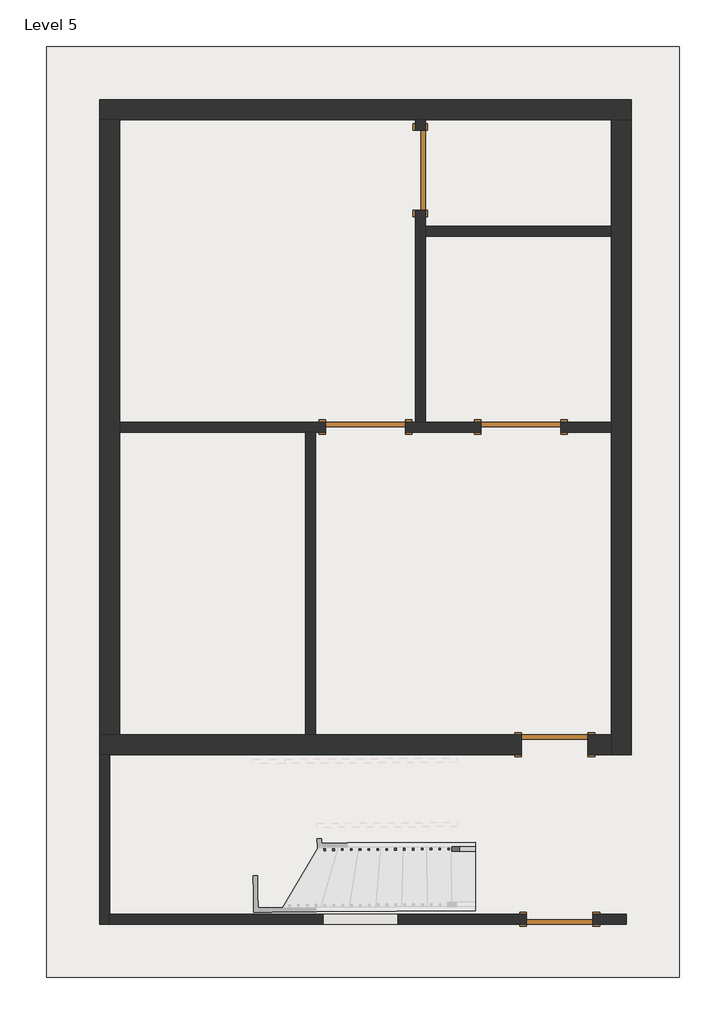
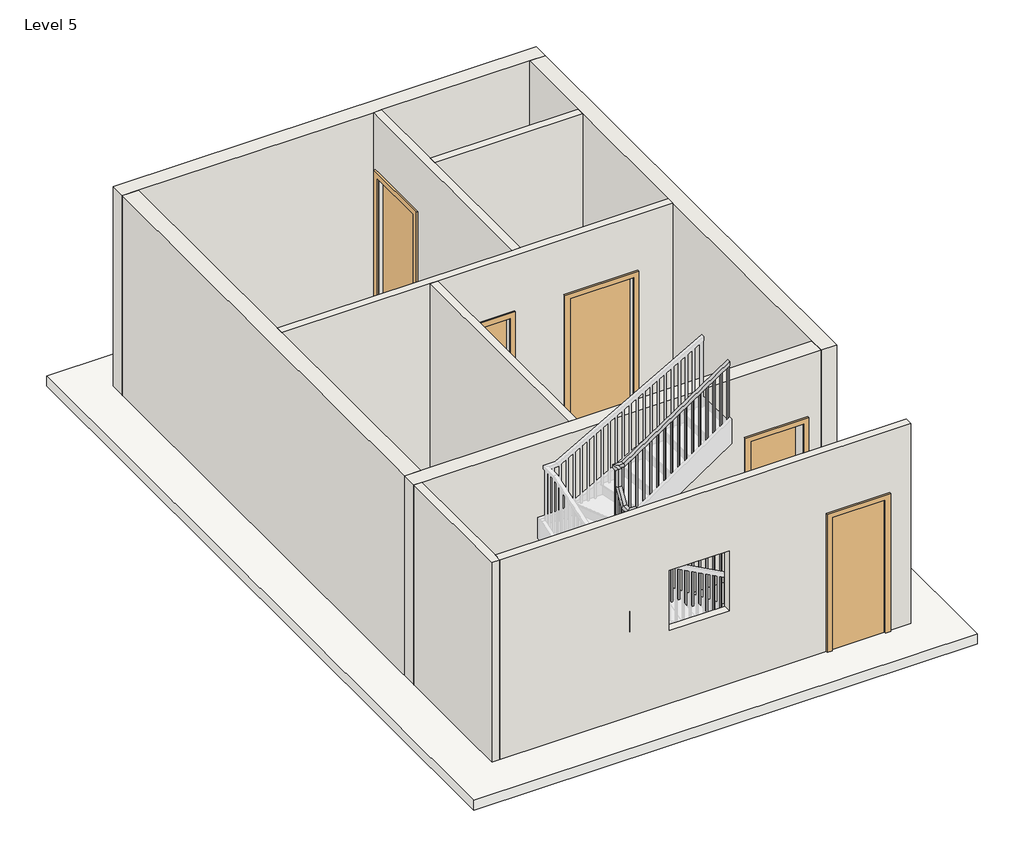
# One storey, part 1 of 2: 10 walls, 5 doors, 1 railing, 1 roof.
"""IFC4 building model written with IfcOpenShell, lengths in millimetres."""

from ifc_helpers import new_model, si_unit, frame, origin, place, context, project, spatial, polyline, outline, extrude, faceted_brep, transform, mapped, element, save
from components import door_a1484949, door_d8f5dbb5, door_e5f9f3c4, door_305aa2a5

model = new_model("IFC4")

# Units and contexts
model_context = context("Model", 3, world=origin())
ifc_project = project(units=[si_unit("LENGTHUNIT", "METRE", prefix="MILLI")], contexts=[model_context])

# Site, building, storey
site = spatial("IfcSite", under=ifc_project)
building = spatial("IfcBuilding", under=site)
storey = spatial("IfcBuildingStorey", under=building, Name="Level 5", Elevation=9601.2)

# Doors
placement = place(None, origin())
door_shape = door_a1484949(model_context)
element("IfcDoor", 1, ObjectType="Single-Flush : 30\" x 80\"", at=placement, inside=storey, context=model_context, shape_type="MappedRepresentation", body=[
    mapped(door_shape, transform((792.5410386, -2372.0109248, 9601.2), x_axis=(1.0, 0.0, 0.0), y_axis=(0.0, 1.0, 0.0), z_axis=(0.0, 0.0, 1.0))),
])
door_2_shape = door_d8f5dbb5(model_context)
element("IfcDoor", 2, ObjectType="Single-Flush : 30\" x 80\"", at=placement, inside=storey, context=model_context, shape_type="MappedRepresentation", body=[
    mapped(door_2_shape, transform((849.6910386, -4372.2609248, 9601.2), x_axis=(-1.0, 0.0, 0.0), y_axis=(0.0, -1.0, 0.0), z_axis=(0.0, 0.0, 1.0))),
])
door_3_shape = door_e5f9f3c4(model_context)
element("IfcDoor", 3, ObjectType="Single-Flush : 36\" x 84\"", at=placement, inside=storey, context=model_context, shape_type="MappedRepresentation", body=[
    mapped(door_3_shape, transform((-750.5089614, 4209.7640752, 9601.2), x_axis=(0.0, -1.0, 0.0), y_axis=(1.0, 0.0, 0.0), z_axis=(0.0, 0.0, 1.0))),
])
door_4_shape = door_305aa2a5(model_context)
element("IfcDoor", 4, ObjectType="Single-Flush : 36\" x 84\"", at=placement, inside=storey, context=model_context, shape_type="MappedRepresentation", body=[
    mapped(door_4_shape, transform((402.0160386, 1266.5390752, 9601.2), x_axis=(-1.0, 0.0, 0.0), y_axis=(0.0, -1.0, 0.0), z_axis=(0.0, 0.0, 1.0))),
])
element("IfcDoor", 5, ObjectType="Single-Flush : 36\" x 84\"", at=placement, inside=storey, context=model_context, shape_type="MappedRepresentation", body=[
    mapped(door_4_shape, transform((-1379.1589614, 1266.5390752, 9601.2), x_axis=(-1.0, 0.0, 0.0), y_axis=(0.0, -1.0, 0.0), z_axis=(0.0, 0.0, 1.0))),
])

# Railing
element("IfcRailing", 6, ObjectType="Handrail - Rectangular", at=placement, inside=storey, context=model_context, shape_type="SolidModel", body=[
    faceted_brep([(-120.3816305, -3590.4209536, 10684.9333333), (-120.3816305, -3590.4209536, 10623.7630107), (-120.6930289, -3539.621908, 10623.7630107), (-120.6930289, -3539.621908, 10684.9333333), (-1854.5612186, -3601.0514854, 11848.2182998), (-1905.3602642, -3601.3628839, 11821.1238978), (-1905.6716627, -3550.5638383, 11821.1238978), (-1854.8726171, -3550.2524399, 11848.2182998), (-1854.5612186, -3601.0514854, 12070.4829276), (-1905.3602642, -3601.3628839, 12019.6829276), (-1905.6716627, -3550.5638383, 12019.6829276), (-1854.8726171, -3550.2524399, 12070.4829276), (-1981.5588325, -3601.8299816, 12070.4829276), (-1981.5588325, -3601.8299816, 12019.6829276), (-1931.0711854, -3550.7195376, 12019.6829276), (-1931.0711854, -3550.7195376, 12070.4829276), (-1982.3373287, -3474.8323677, 12070.4829276), (-1982.5128182, -3446.2044317, 12019.6829276), (-1931.7137726, -3445.8930332, 12019.6829276), (-1931.5382832, -3474.5209692, 12070.4829276), (-1983.1158249, -3347.8347538, 12280.2434812), (-1983.4272234, -3297.0357082, 12266.0632575), (-1932.6281778, -3296.7243097, 12266.0632575), (-1932.3167793, -3347.5233553, 12280.2434812), (-1983.1158249, -3347.8347538, 12551.6951436), (-1983.4272234, -3297.0357082, 12500.8951436), (-1932.6281778, -3296.7243097, 12500.8951436), (-1932.3167793, -3347.5233553, 12551.6951436), (-1983.8943211, -3220.8371398, 12551.6951436), (-1983.8943211, -3220.8371398, 12500.8951436), (-1932.783877, -3271.3247869, 12500.8951436), (-1932.783877, -3271.3247869, 12551.6951436), (-1856.8967072, -3220.0586437, 12551.6951436), (-1841.6341703, -3219.9650842, 12500.8951436), (-1841.3227719, -3270.7641298, 12500.8951436), (-1856.5853087, -3270.8576892, 12551.6951436), (-324.9523945, -3210.6678153, 13563.6), (-324.6409961, -3261.4668609, 13563.6), (-324.6409961, -3261.4668609, 13502.7185401), (-324.9523945, -3210.6678153, 13502.7185401)], [[[0, 1, 2, 3]], [[1, 0, 4, 5]], [[2, 1, 5, 6]], [[3, 2, 6, 7]], [[0, 3, 7, 4]], [[5, 4, 8, 9]], [[6, 5, 9, 10]], [[7, 6, 10, 11]], [[4, 7, 11, 8]], [[9, 8, 12, 13]], [[10, 9, 13, 14]], [[11, 10, 14, 15]], [[8, 11, 15, 12]], [[13, 12, 16, 17]], [[14, 13, 17, 18]], [[15, 14, 18, 19]], [[12, 15, 19, 16]], [[17, 16, 20, 21]], [[18, 17, 21, 22]], [[19, 18, 22, 23]], [[16, 19, 23, 20]], [[21, 20, 24, 25]], [[22, 21, 25, 26]], [[23, 22, 26, 27]], [[20, 23, 27, 24]], [[25, 24, 28, 29]], [[26, 25, 29, 30]], [[27, 26, 30, 31]], [[24, 27, 31, 28]], [[29, 28, 32, 33]], [[30, 29, 33, 34]], [[31, 30, 34, 35]], [[28, 31, 35, 32]], [[36, 37, 38, 39]], [[33, 32, 36, 39]], [[34, 33, 39, 38]], [[35, 34, 38, 37]], [[32, 35, 37, 36]]]),
    extrude(outline(polyline([(222.3085098, -19.05), (234.8914903, 0.0), (1246.1854534, 0.0), (1246.1854534, -19.05), (222.3085098, -19.05)])), frame((-342.2360746, -3245.6994205, 13726.0521201), z_axis=(-0.00612989118043648, 0.9999812120405643, 0.0), x_axis=(0.0, 0.0, -1.0)), (0.0, 0.0, 1.0), 19.05),
    extrude(outline(polyline([(222.3085098, -19.0499999), (234.8914902, 0.0), (1179.0762243, 0.0), (1179.0762243, -19.0499999), (222.3085098, -19.0499999)])), frame((-443.8341657, -3246.3222175, 13658.942891), z_axis=(-0.00612989118043648, 0.9999812120405643, 0.0), x_axis=(0.0, 0.0, -1.0)), (0.0, 0.0, 1.0), 19.05),
    extrude(outline(polyline([(222.3085098, -19.05), (234.8914902, 0.0), (1111.9669952, 0.0), (1111.9669952, -19.05), (222.3085098, -19.05)])), frame((-545.4322569, -3246.9450144, 13591.8336619), z_axis=(-0.00612989118043648, 0.9999812120405643, 0.0), x_axis=(0.0, 0.0, -1.0)), (0.0, 0.0, 1.0), 19.05),
    extrude(outline(polyline([(222.3085098, -19.05), (234.8914902, 0.0), (1214.1910995, 0.0), (1214.1910995, -19.05), (222.3085098, -19.05)])), frame((-647.030348, -3247.5678114, 13524.7244328), z_axis=(-0.00612989118043648, 0.9999812120405643, 0.0), x_axis=(0.0, 0.0, -1.0)), (0.0, 0.0, 1.0), 19.05),
    extrude(outline(polyline([(222.3085098, -19.05), (234.8914902, 0.0), (1147.0818704, 0.0), (1147.0818704, -19.05), (222.3085098, -19.05)])), frame((-748.6284392, -3248.1906083, 13457.6152037), z_axis=(-0.00612989118043648, 0.9999812120405643, 0.0), x_axis=(0.0, 0.0, -1.0)), (0.0, 0.0, 1.0), 19.05),
    extrude(outline(polyline([(222.3085098, -19.05), (234.8914902, 0.0), (1079.9726413, 0.0), (1079.9726413, -19.05), (222.3085098, -19.05)])), frame((-850.2265303, -3248.8134053, 13390.5059746), z_axis=(-0.00612989118043648, 0.9999812120405643, 0.0), x_axis=(0.0, 0.0, -1.0)), (0.0, 0.0, 1.0), 19.05),
    extrude(outline(polyline([(222.3085098, -19.05), (234.8914902, 0.0), (1182.1967455, 0.0), (1182.1967455, -19.05), (222.3085098, -19.05)])), frame((-951.8246215, -3249.4362022, 13323.3967455), z_axis=(-0.00612989118043648, 0.9999812120405643, 0.0), x_axis=(0.0, 0.0, -1.0)), (0.0, 0.0, 1.0), 19.05),
    extrude(outline(polyline([(222.3085097, -19.05), (234.8914902, 0.0), (1115.0875164, 0.0), (1115.0875164, -19.05), (222.3085097, -19.05)])), frame((-1053.4227126, -3250.0589992, 13256.2875164), z_axis=(-0.00612989118043648, 0.9999812120405643, 0.0), x_axis=(0.0, 0.0, -1.0)), (0.0, 0.0, 1.0), 19.05),
    extrude(outline(polyline([(222.3085097, -19.0499999), (234.8914902, 0.0), (1047.9782873, 0.0), (1047.9782873, -19.0499999), (222.3085097, -19.0499999)])), frame((-1155.0208037, -3250.6817961, 13189.1782873), z_axis=(-0.00612989118043648, 0.9999812120405643, 0.0), x_axis=(0.0, 0.0, -1.0)), (0.0, 0.0, 1.0), 19.05),
    extrude(outline(polyline([(222.3085097, -19.05), (234.8914902, 0.0), (1150.2023915, 0.0), (1150.2023915, -19.05), (222.3085097, -19.05)])), frame((-1256.6188949, -3251.304593, 13122.0690582), z_axis=(-0.00612989118043648, 0.9999812120405643, 0.0), x_axis=(0.0, 0.0, -1.0)), (0.0, 0.0, 1.0), 19.05),
    extrude(outline(polyline([(222.3085098, -19.05), (234.8914903, 0.0), (1083.0931625, 0.0), (1083.0931625, -19.05), (222.3085098, -19.05)])), frame((-1358.216986, -3251.92739, 13054.9598292), z_axis=(-0.00612989118043648, 0.9999812120405643, 0.0), x_axis=(0.0, 0.0, -1.0)), (0.0, 0.0, 1.0), 19.05),
    extrude(outline(polyline([(222.3085098, -19.05), (234.8914903, 0.0), (1185.3172668, 0.0), (1185.3172668, -19.05), (222.3085098, -19.05)])), frame((-1459.8150772, -3252.5501869, 12987.8506001), z_axis=(-0.00612989118043648, 0.9999812120405643, 0.0), x_axis=(0.0, 0.0, -1.0)), (0.0, 0.0, 1.0), 19.05),
    extrude(outline(polyline([(222.3085098, -19.05), (234.8914903, 0.0), (1118.2080377, 0.0), (1118.2080377, -19.05), (222.3085098, -19.05)])), frame((-1561.4131683, -3253.1729839, 12920.741371), z_axis=(-0.00612989118043648, 0.9999812120405643, 0.0), x_axis=(0.0, 0.0, -1.0)), (0.0, 0.0, 1.0), 19.05),
    extrude(outline(polyline([(222.3085098, -19.05), (234.8914902, 0.0), (1051.0988086, 0.0), (1051.0988086, -19.05), (222.3085098, -19.05)])), frame((-1663.0112595, -3253.7957808, 12853.6321419), z_axis=(-0.00612989118043648, 0.9999812120405643, 0.0), x_axis=(0.0, 0.0, -1.0)), (0.0, 0.0, 1.0), 19.05),
    extrude(outline(polyline([(222.3085098, -19.05), (234.8914902, 0.0), (1153.3229128, 0.0), (1153.3229128, -19.05), (222.3085098, -19.05)])), frame((-1764.6093506, -3254.4185778, 12786.5229128), z_axis=(-0.00612989118043648, 0.9999812120405643, 0.0), x_axis=(0.0, 0.0, -1.0)), (0.0, 0.0, 1.0), 19.05),
    extrude(outline(polyline([(222.3085098, -19.05), (234.8914902, 0.0), (1086.2136837, 0.0), (1086.2136837, -19.05), (222.3085098, -19.05)])), frame((-1866.2074418, -3255.0413747, 12719.4136837), z_axis=(-0.00612989118043648, 0.9999812120405643, 0.0), x_axis=(0.0, 0.0, -1.0)), (0.0, 0.0, 1.0), 19.05),
    extrude(outline(polyline([(-1948.6001916, -3280.94692), (-1967.6498337, -3281.0636944), (-1967.7666081, -3262.0140523), (-1948.716966, -3261.8972779), (-1948.6001916, -3280.94692)])), frame((0.0, 0.0, 11463.8666667), z_axis=(0.0, 0.0, 1.0), x_axis=(1.0, 0.0, 0.0)), (0.0, 0.0, 1.0), 1037.0284769),
    extrude(outline(polyline([(244.3320415, -19.05), (212.8679585, 0.0), (1074.2735921, 0.0), (1074.2735921, -19.05), (244.3320415, -19.05)])), frame((-1967.1438111, -3363.6121435, 12368.8069254), z_axis=(0.9999812120405644, 0.006129891180436036, 0.0), x_axis=(0.0, 0.0, -1.0)), (0.0, 0.0, 1.0), 19.05),
    extrude(outline(polyline([(244.3320415, -19.05), (212.8679585, 0.0), (1075.7984825, 0.0), (1075.7984825, -19.05), (244.3320415, -19.05)])), frame((-1966.5210142, -3465.2102346, 12200.9984825), z_axis=(0.9999812120405644, 0.006129891180436036, 0.0), x_axis=(0.0, 0.0, -1.0)), (0.0, 0.0, 1.0), 19.05),
    extrude(outline(polyline([(-1939.8365364, -3566.6485675), (-1939.719762, -3585.6982096), (-1958.7694041, -3585.814984), (-1958.8861785, -3566.7653419), (-1939.8365364, -3566.6485675)])), frame((0.0, 0.0, 10955.8666667), z_axis=(0.0, 0.0, 1.0), x_axis=(1.0, 0.0, 0.0)), (0.0, 0.0, 1.0), 1063.816261),
    extrude(outline(polyline([(234.9892351, -19.05), (222.2107648, 0.0), (1224.4109792, 0.0), (1224.4109792, -19.05), (234.9892351, -19.05)])), frame((-1857.171313, -3585.1921871, 12010.9443125), z_axis=(-0.006129891180436334, 0.9999812120405643, 0.0), x_axis=(0.0, 0.0, -1.0)), (0.0, 0.0, 1.0), 19.05),
    extrude(outline(polyline([(234.9892352, -19.05), (222.2107649, 0.0), (1156.259138, 0.0), (1156.259138, -19.05), (234.9892352, -19.05)])), frame((-1755.5732218, -3584.5693901, 11942.7924713), z_axis=(-0.006129891180436334, 0.9999812120405643, 0.0), x_axis=(0.0, 0.0, -1.0)), (0.0, 0.0, 1.0), 19.05),
    extrude(outline(polyline([(234.9892351, -19.05), (222.2107649, 0.0), (1257.44063, 0.0), (1257.44063, -19.05), (234.9892351, -19.05)])), frame((-1653.9751307, -3583.9465932, 11874.64063), z_axis=(-0.006129891180436334, 0.9999812120405643, 0.0), x_axis=(0.0, 0.0, -1.0)), (0.0, 0.0, 1.0), 19.05),
    extrude(outline(polyline([(234.9892351, -19.05), (222.2107649, 0.0), (1189.2887887, 0.0), (1189.2887887, -19.05), (234.9892351, -19.05)])), frame((-1552.3770395, -3583.3237962, 11806.4887887), z_axis=(-0.006129891180436334, 0.9999812120405643, 0.0), x_axis=(0.0, 0.0, -1.0)), (0.0, 0.0, 1.0), 19.05),
    extrude(outline(polyline([(234.9892351, -19.05), (222.2107649, 0.0), (1290.4702807, 0.0), (1290.4702807, -19.05), (234.9892351, -19.05)])), frame((-1450.7789484, -3582.7009993, 11738.3369474), z_axis=(-0.006129891180436334, 0.9999812120405643, 0.0), x_axis=(0.0, 0.0, -1.0)), (0.0, 0.0, 1.0), 19.05),
    extrude(outline(polyline([(234.9892351, -19.0499999), (222.2107649, 0.0), (1222.3184394, 0.0), (1222.3184394, -19.0499999), (234.9892351, -19.0499999)])), frame((-1349.1808572, -3582.0782024, 11670.1851061), z_axis=(-0.006129891180436334, 0.9999812120405643, 0.0), x_axis=(0.0, 0.0, -1.0)), (0.0, 0.0, 1.0), 19.05),
    extrude(outline(polyline([(234.9892351, -19.05), (222.2107648, 0.0), (1154.1665981, 0.0), (1154.1665981, -19.05), (234.9892351, -19.05)])), frame((-1247.5827661, -3581.4554054, 11602.0332648), z_axis=(-0.006129891180436334, 0.9999812120405643, 0.0), x_axis=(0.0, 0.0, -1.0)), (0.0, 0.0, 1.0), 19.05),
    extrude(outline(polyline([(234.9892352, -19.05), (222.2107649, 0.0), (1255.3480903, 0.0), (1255.3480903, -19.05), (234.9892352, -19.05)])), frame((-1145.984675, -3580.8326085, 11533.8814236), z_axis=(-0.006129891180436334, 0.9999812120405643, 0.0), x_axis=(0.0, 0.0, -1.0)), (0.0, 0.0, 1.0), 19.05),
    extrude(outline(polyline([(234.9892351, -19.05), (222.2107649, 0.0), (1187.196249, 0.0), (1187.196249, -19.05), (234.9892351, -19.05)])), frame((-1044.3865838, -3580.2098115, 11465.7295823), z_axis=(-0.006129891180436334, 0.9999812120405643, 0.0), x_axis=(0.0, 0.0, -1.0)), (0.0, 0.0, 1.0), 19.05),
    extrude(outline(polyline([(234.9892351, -19.05), (222.2107649, 0.0), (1288.377741, 0.0), (1288.377741, -19.05), (234.9892351, -19.05)])), frame((-942.7884927, -3579.5870146, 11397.577741), z_axis=(-0.006129891180436334, 0.9999812120405643, 0.0), x_axis=(0.0, 0.0, -1.0)), (0.0, 0.0, 1.0), 19.05),
    extrude(outline(polyline([(234.9892351, -19.05), (222.2107649, 0.0), (1220.2258997, 0.0), (1220.2258997, -19.05), (234.9892351, -19.05)])), frame((-841.1904015, -3578.9642176, 11329.4258997), z_axis=(-0.006129891180436334, 0.9999812120405643, 0.0), x_axis=(0.0, 0.0, -1.0)), (0.0, 0.0, 1.0), 19.05),
    extrude(outline(polyline([(234.9892351, -19.05), (222.2107649, 0.0), (1152.0740584, 0.0), (1152.0740584, -19.05), (234.9892351, -19.05)])), frame((-739.5923104, -3578.3414207, 11261.2740584), z_axis=(-0.006129891180436334, 0.9999812120405643, 0.0), x_axis=(0.0, 0.0, -1.0)), (0.0, 0.0, 1.0), 19.05),
    extrude(outline(polyline([(234.9892351, -19.0499999), (222.2107648, 0.0), (1253.2555504, 0.0), (1253.2555504, -19.0499999), (234.9892351, -19.0499999)])), frame((-637.9942192, -3577.7186237, 11193.1222171), z_axis=(-0.006129891180436334, 0.9999812120405643, 0.0), x_axis=(0.0, 0.0, -1.0)), (0.0, 0.0, 1.0), 19.05),
    extrude(outline(polyline([(234.9892352, -19.05), (222.2107649, 0.0), (1185.1037092, 0.0), (1185.1037092, -19.05), (234.9892352, -19.05)])), frame((-536.3961281, -3577.0958268, 11124.9703759), z_axis=(-0.006129891180436334, 0.9999812120405643, 0.0), x_axis=(0.0, 0.0, -1.0)), (0.0, 0.0, 1.0), 19.05),
    extrude(outline(polyline([(234.9892351, -19.05), (222.2107649, 0.0), (1116.9518679, 0.0), (1116.9518679, -19.05), (234.9892351, -19.05)])), frame((-434.798037, -3576.4730299, 11056.8185346), z_axis=(-0.006129891180436334, 0.9999812120405643, 0.0), x_axis=(0.0, 0.0, -1.0)), (0.0, 0.0, 1.0), 19.05),
    extrude(outline(polyline([(234.9892351, -19.05), (222.2107649, 0.0), (1218.13336, 0.0), (1218.13336, -19.05), (234.9892351, -19.05)])), frame((-333.1999458, -3575.8502329, 10988.6666933), z_axis=(-0.006129891180436334, 0.9999812120405643, 0.0), x_axis=(0.0, 0.0, -1.0)), (0.0, 0.0, 1.0), 19.05),
    extrude(outline(polyline([(234.9892351, -19.05), (222.2107649, 0.0), (1149.9815187, 0.0), (1149.9815187, -19.05), (234.9892351, -19.05)])), frame((-231.6018547, -3575.227436, 10920.514852), z_axis=(-0.006129891180436334, 0.9999812120405643, 0.0), x_axis=(0.0, 0.0, -1.0)), (0.0, 0.0, 1.0), 19.05),
    extrude(outline(polyline([(-1948.7558908, -3255.5473972), (-1967.8055329, -3255.6641716), (-1967.9223073, -3236.6145296), (-1948.8726652, -3236.4977551), (-1948.7558908, -3255.5473972)])), frame((0.0, 0.0, 11463.8666667), z_axis=(0.0, 0.0, 1.0), x_axis=(1.0, 0.0, 0.0)), (0.0, 0.0, 1.0), 1037.0284769),
    extrude(outline(polyline([(-1946.8485752, -3566.6915513), (-1946.7318007, -3585.7411934), (-1965.7814428, -3585.8579679), (-1965.8982173, -3566.8083258), (-1946.8485752, -3566.6915513)])), frame((0.0, 0.0, 10955.8666667), z_axis=(0.0, 0.0, 1.0), x_axis=(1.0, 0.0, 0.0)), (0.0, 0.0, 1.0), 1063.816261),
    extrude(outline(polyline([(222.3085098, -19.05), (234.8914902, 0.0), (1245.1603832, 0.0), (1245.1603832, -19.05), (222.3085098, -19.05)])), frame((-343.7879502, -3245.7089335, 13725.0270499), z_axis=(-0.00612989118043648, 0.9999812120405643, 0.0), x_axis=(0.0, 0.0, -1.0)), (0.0, 0.0, 1.0), 19.05),
    extrude(outline(polyline([(234.9892351, -19.05), (222.2107648, 0.0), (1088.2189125, 0.0), (1088.2189125, -19.05), (234.9892351, -19.05)])), frame((-139.5285846, -3574.6630262, 10858.7522458), z_axis=(-0.006129891180436334, 0.9999812120405643, 0.0), x_axis=(0.0, 0.0, -1.0)), (0.0, 0.0, 1.0), 19.05),
])

# Roof
element("IfcRoof", 7, ObjectType="Generic - 12\"", at=placement, inside=storey, context=model_context, shape_type="SweptSolid", body=[
    extrude(outline(polyline([(-5036.7589614, 5628.9890752), (2221.2910386, 5628.9890752), (2221.2910386, -5039.0109248), (-5036.7589614, -5039.0109248), (-5036.7589614, 5628.9890752)])), frame((0.0, 0.0, 9448.8), z_axis=(0.0, 0.0, 1.0), x_axis=(1.0, 0.0, 0.0)), (0.0, 0.0, 1.0), 152.4),
])

# Walls
element("IfcWall", 8, ObjectType="4.5\"", at=placement, inside=storey, context=model_context, shape_type="Brep", body=[
    faceted_brep([(-807.6589614, 3752.5640752, 11734.8), (-807.6589614, 3752.5640752, 9601.2), (-807.6589614, 1323.6890752, 9601.2), (-807.6589614, 1323.6890752, 12649.2), (-807.6589614, 4790.7890752, 12649.2), (-807.6589614, 4790.7890752, 9601.2), (-807.6589614, 4666.9640752, 9601.2), (-807.6589614, 4666.9640752, 11734.8), (-693.3589614, 1323.6890752, 9601.2), (-693.3589614, 3457.2890752, 9601.2), (-693.3589614, 3571.5890752, 9601.2), (-693.3589614, 3752.5640752, 9601.2), (-693.3589614, 3752.5640752, 11734.8), (-693.3589614, 4666.9640752, 11734.8), (-693.3589614, 4666.9640752, 9601.2), (-693.3589614, 4790.7890752, 9601.2), (-693.3589614, 4790.7890752, 12649.2), (-693.3589614, 3571.5890752, 12649.2), (-693.3589614, 3457.2890752, 12649.2), (-693.3589614, 1323.6890752, 12649.2)], [[[0, 1, 2, 3, 4, 5, 6, 7]], [[8, 9, 10, 11, 12, 13, 14, 15, 16, 17, 18, 19]], [[6, 5, 15, 14]], [[2, 1, 11, 10, 9, 8]], [[5, 4, 16, 15]], [[3, 2, 8, 19]], [[12, 11, 1, 0]], [[13, 12, 0, 7]], [[14, 13, 7, 6]], [[4, 3, 19, 18, 17, 16]]]),
])
element("IfcWall", 9, ObjectType="4.5\"", at=placement, inside=storey, context=model_context, shape_type="SweptSolid", body=[
    extrude(outline(polyline([(-693.3589614, 3571.5890752), (1440.2410386, 3571.5890752), (1440.2410386, 3457.2890752), (-693.3589614, 3457.2890752), (-693.3589614, 3571.5890752)])), frame((0.0, 0.0, 9601.2), z_axis=(0.0, 0.0, 1.0), x_axis=(1.0, 0.0, 0.0)), (0.0, 0.0, 1.0), 3048.0),
])
element("IfcWall", 10, ObjectType="4.5\"", at=placement, inside=storey, context=model_context, shape_type="Brep", body=[
    faceted_brep([(-4198.5589614, 1209.3890752, 9601.2), (-2064.9589614, 1209.3890752, 9601.2), (-1950.6589614, 1209.3890752, 9601.2), (-1836.3589614, 1209.3890752, 9601.2), (-1836.3589614, 1209.3890752, 11734.8), (-921.9589614, 1209.3890752, 11734.8), (-921.9589614, 1209.3890752, 9601.2), (-55.1839614, 1209.3890752, 9601.2), (-55.1839614, 1209.3890752, 11734.8), (859.2160386, 1209.3890752, 11734.8), (859.2160386, 1209.3890752, 9601.2), (1440.2410386, 1209.3890752, 9601.2), (1440.2410386, 1209.3890752, 12649.2), (-1950.6589614, 1209.3890752, 12649.2), (-2064.9589614, 1209.3890752, 12649.2), (-4198.5589614, 1209.3890752, 12649.2), (-1836.3589614, 1323.6890752, 11734.8), (-1836.3589614, 1323.6890752, 9601.2), (-4198.5589614, 1323.6890752, 9601.2), (-4198.5589614, 1323.6890752, 12649.2), (-807.6589614, 1323.6890752, 12649.2), (-693.3589614, 1323.6890752, 12649.2), (1440.2410386, 1323.6890752, 12649.2), (1440.2410386, 1323.6890752, 9601.2), (859.2160386, 1323.6890752, 9601.2), (859.2160386, 1323.6890752, 11734.8), (-55.1839614, 1323.6890752, 11734.8), (-55.1839614, 1323.6890752, 9601.2), (-693.3589614, 1323.6890752, 9601.2), (-807.6589614, 1323.6890752, 9601.2), (-921.9589614, 1323.6890752, 9601.2), (-921.9589614, 1323.6890752, 11734.8)], [[[0, 1, 2, 3, 4, 5, 6, 7, 8, 9, 10, 11, 12, 13, 14, 15]], [[16, 17, 18, 19, 20, 21, 22, 23, 24, 25, 26, 27, 28, 29, 30, 31]], [[24, 23, 11, 10]], [[18, 17, 3, 2, 1, 0]], [[30, 29, 28, 27, 7, 6]], [[12, 11, 23, 22]], [[0, 15, 19, 18]], [[8, 7, 27, 26]], [[9, 8, 26, 25]], [[10, 9, 25, 24]], [[4, 3, 17, 16]], [[5, 4, 16, 31]], [[6, 5, 31, 30]], [[15, 14, 13, 12, 22, 21, 20, 19]]]),
])
element("IfcWall", 11, ObjectType="4.5\"", at=placement, inside=storey, context=model_context, shape_type="SweptSolid", body=[
    extrude(outline(polyline([(-2064.9589614, -2257.7109248), (-2064.9589614, 1209.3890752), (-1950.6589614, 1209.3890752), (-1950.6589614, -2257.7109248), (-2064.9589614, -2257.7109248)])), frame((0.0, 0.0, 9601.2), z_axis=(0.0, 0.0, 1.0), x_axis=(1.0, 0.0, 0.0)), (0.0, 0.0, 1.0), 3048.0),
])
element("IfcWall", 12, ObjectType="4.5\"", at=placement, inside=storey, context=model_context, shape_type="Brep", body=[
    faceted_brep([(-4427.1589614, -2486.3109248, 9601.2), (-4427.1589614, -4429.4109248, 9601.2), (-4427.1589614, -4429.4109248, 12649.2), (-4427.1589614, -2486.3109248, 12649.2), (-4312.8589614, -2486.3109248, 9601.2), (-4312.8589614, -2486.3109248, 12649.2), (-4312.8589614, -4315.1109248, 12649.2), (-4312.8589614, -4429.4109248, 12649.2), (-4312.8589614, -4429.4109248, 9601.2), (-4312.8589614, -4315.1109248, 9601.2)], [[[0, 1, 2, 3]], [[4, 5, 6, 7, 8, 9]], [[1, 0, 4, 9, 8]], [[3, 2, 7, 6, 5]], [[0, 3, 5, 4]], [[2, 1, 8, 7]]]),
])
element("IfcWall", 13, ObjectType="4.5\"", at=placement, inside=storey, context=model_context, shape_type="SweptSolid", body=[
    extrude(outline(polyline([(9601.2, -4312.8589614), (9601.2, 468.6910386), (11633.2, 468.6910386), (11633.2, 1230.6910386), (9601.2, 1230.6910386), (9601.2, 1611.6910386), (12649.2, 1611.6910386), (12649.2, -4312.8589614), (9601.2, -4312.8589614)]), holes=[polyline([(11626.5390194, -1868.1089614), (11626.5390194, -1004.5089614), (10712.1390194, -1004.5089614), (10712.1390194, -1868.1089614), (11626.5390194, -1868.1089614)])]), frame((0.0, -4429.4109248, 0.0), z_axis=(0.0, 1.0, 0.0), x_axis=(0.0, 0.0, 1.0)), (0.0, 0.0, 1.0), 114.3),
])
element("IfcWall", 14, ObjectType="9\"", at=placement, inside=storey, context=model_context, shape_type="Brep", body=[
    faceted_brep([(-4427.1589614, 4790.7890752, 9601.2), (-4198.5589614, 4790.7890752, 9601.2), (-807.6589614, 4790.7890752, 9601.2), (-693.3589614, 4790.7890752, 9601.2), (1440.2410386, 4790.7890752, 9601.2), (1668.8410386, 4790.7890752, 9601.2), (1668.8410386, 4790.7890752, 12649.2), (1440.2410386, 4790.7890752, 12649.2), (-693.3589614, 4790.7890752, 12649.2), (-807.6589614, 4790.7890752, 12649.2), (-4198.5589614, 4790.7890752, 12649.2), (-4427.1589614, 4790.7890752, 12649.2), (-4427.1589614, 5019.3890752, 9601.2), (-4427.1589614, 5019.3890752, 12649.2), (1668.8410386, 5019.3890752, 12649.2), (1668.8410386, 5019.3890752, 9601.2)], [[[0, 1, 2, 3, 4, 5, 6, 7, 8, 9, 10, 11]], [[12, 13, 14, 15]], [[5, 4, 3, 2, 1, 0, 12, 15]], [[6, 5, 15, 14]], [[0, 11, 13, 12]], [[11, 10, 9, 8, 7, 6, 14, 13]]]),
])
element("IfcWall", 15, ObjectType="9\"", at=placement, inside=storey, context=model_context, shape_type="Brep", body=[
    faceted_brep([(1440.2410386, 4790.7890752, 9601.2), (1440.2410386, 3571.5890752, 9601.2), (1440.2410386, 3457.2890752, 9601.2), (1440.2410386, 1323.6890752, 9601.2), (1440.2410386, 1209.3890752, 9601.2), (1440.2410386, -2257.7109248, 9601.2), (1440.2410386, -2486.3109248, 9601.2), (1440.2410386, -2486.3109248, 12649.2), (1440.2410386, -2257.7109248, 12649.2), (1440.2410386, 1209.3890752, 12649.2), (1440.2410386, 1323.6890752, 12649.2), (1440.2410386, 3457.2890752, 12649.2), (1440.2410386, 3571.5890752, 12649.2), (1440.2410386, 4790.7890752, 12649.2), (1668.8410386, 4790.7890752, 9601.2), (1668.8410386, 4790.7890752, 12649.2), (1668.8410386, -2486.3109248, 12649.2), (1668.8410386, -2486.3109248, 9601.2)], [[[0, 1, 2, 3, 4, 5, 6, 7, 8, 9, 10, 11, 12, 13]], [[14, 15, 16, 17]], [[6, 5, 4, 3, 2, 1, 0, 14, 17]], [[0, 13, 15, 14]], [[7, 6, 17, 16]], [[13, 12, 11, 10, 9, 8, 7, 16, 15]]]),
])
element("IfcWall", 16, ObjectType="9\"", at=placement, inside=storey, context=model_context, shape_type="Brep", body=[
    faceted_brep([(1440.2410386, -2257.7109248, 9601.2), (1173.5410386, -2257.7109248, 9601.2), (1173.5410386, -2257.7109248, 11633.2), (411.5410386, -2257.7109248, 11633.2), (411.5410386, -2257.7109248, 9601.2), (-1950.6589614, -2257.7109248, 9601.2), (-2064.9589614, -2257.7109248, 9601.2), (-4198.5589614, -2257.7109248, 9601.2), (-4427.1589614, -2257.7109248, 9601.2), (-4427.1589614, -2257.7109248, 12649.2), (-4198.5589614, -2257.7109248, 12649.2), (-2064.9589614, -2257.7109248, 12649.2), (-1950.6589614, -2257.7109248, 12649.2), (1440.2410386, -2257.7109248, 12649.2), (1173.5410386, -2486.3109248, 11633.2), (1173.5410386, -2486.3109248, 9601.2), (1440.2410386, -2486.3109248, 9601.2), (1440.2410386, -2486.3109248, 12649.2), (-4312.8589614, -2486.3109248, 12649.2), (-4427.1589614, -2486.3109248, 12649.2), (-4427.1589614, -2486.3109248, 9601.2), (-4312.8589614, -2486.3109248, 9601.2), (411.5410386, -2486.3109248, 9601.2), (411.5410386, -2486.3109248, 11633.2)], [[[0, 1, 2, 3, 4, 5, 6, 7, 8, 9, 10, 11, 12, 13]], [[14, 15, 16, 17, 18, 19, 20, 21, 22, 23]], [[16, 15, 1, 0]], [[22, 21, 20, 8, 7, 6, 5, 4]], [[0, 13, 17, 16]], [[9, 8, 20, 19]], [[2, 1, 15, 14]], [[3, 2, 14, 23]], [[4, 3, 23, 22]], [[13, 12, 11, 10, 9, 19, 18, 17]]]),
])
element("IfcWall", 17, ObjectType="9\"", at=placement, inside=storey, context=model_context, shape_type="Brep", body=[
    faceted_brep([(-4198.5589614, -2257.7109248, 9601.2), (-4198.5589614, 1209.3890752, 9601.2), (-4198.5589614, 1323.6890752, 9601.2), (-4198.5589614, 4790.7890752, 9601.2), (-4198.5589614, 4790.7890752, 12649.2), (-4198.5589614, 1323.6890752, 12649.2), (-4198.5589614, 1209.3890752, 12649.2), (-4198.5589614, -2257.7109248, 12649.2), (-4427.1589614, -2257.7109248, 9601.2), (-4427.1589614, -2257.7109248, 12649.2), (-4427.1589614, 4790.7890752, 12649.2), (-4427.1589614, 4790.7890752, 9601.2)], [[[0, 1, 2, 3, 4, 5, 6, 7]], [[8, 9, 10, 11]], [[3, 2, 1, 0, 8, 11]], [[0, 7, 9, 8]], [[4, 3, 11, 10]], [[7, 6, 5, 4, 10, 9]]]),
])

save(model, "model.ifc")

# Revit data of these elements
# Type "Single-Flush : 30\" x 80\""
#   Type Mark = "5"
#   Construction Type Id = "MDOOR"
#   Assembly Code = "C1020"
#   Analytic Construction = "Metal"
#   Thickness = 0' - 2"
#   Heat Transfer Coefficient (U) = 0.651978 BTU/(h·ft²·°F)
#   Height = 6' - 8"
#   Trim Projection Ext = 0' - 1"
#   Trim Projection Int = 0' - 1"
#   Trim Width = 0' - 3"
#   Width = 2' - 6"
#   Define Thermal Properties by = 1
#   Define Thermal Properties by = 1
#   Door Material = Door - Panel
#   Frame Material = Door - Frame
#   Visual Light Transmittance = 0
#   Solar Heat Gain Coefficient = 0
#   Function = (empty or 0)
#   Wall Closure = (empty or 0)
# Type "Single-Flush : 36\" x 84\""
#   Type Mark = "1"
#   Construction Type Id = "MDOOR"
#   Assembly Code = "C1020"
#   Analytic Construction = "Metal"
#   Thickness = 0' - 2"
#   Heat Transfer Coefficient (U) = 0.651978 BTU/(h·ft²·°F)
#   Height = 7' - 0"
#   Trim Projection Ext = 0' - 1"
#   Trim Projection Int = 0' - 1"
#   Trim Width = 0' - 3"
#   Width = 3' - 0"
#   Define Thermal Properties by = 1
#   Define Thermal Properties by = 1
#   Door Material = Door - Panel
#   Frame Material = Door - Frame
#   Visual Light Transmittance = 0
#   Solar Heat Gain Coefficient = 0
#   Function = (empty or 0)
#   Wall Closure = (empty or 0)
# Type "Handrail - Rectangular"
#   Assembly Code = "C2010400"
#   built-in parameter 1008612 = 0.0416667 (stored number, unit not read)
#   built-in parameter 1008611 = 0.0416667 (stored number, unit not read)
#   built-in parameter 1008609 = 0.333333 (stored number, unit not read)
#   built-in parameter 1008604 = 0.166667 (stored number, unit not read)
#   built-in parameter 1008603 = 0.166667 (stored number, unit not read)
#   Railing Height = 3' - 0"
#   built-in parameter 1008630 = 2
#   built-in parameter 1008610 = 2
#   built-in parameter 1008618 = Baluster - Square : 3/4"
# Type "Generic - 12\""
#   Assembly Code = "B1020"
#   Layers, outside or top first: 0' - 6" no material (function 1)
# Type "4.5\""
#   Assembly Code = "B2010"
#   Layers, outside or top first: 0' - 4 1/2" no material (function 1)
# Type "9\""
#   Assembly Code = "B2010"
#   Layers, outside or top first: 0' - 9" no material (function 1)
# Elements 1, 2 (IfcDoor, "Single-Flush : 30\" x 80\"")
#   Phase Created = New Construction
#   Materials on its faces: "Door - Frame", "Door - Panel"
# Elements 3, 4, 5 (IfcDoor, "Single-Flush : 36\" x 84\"")
#   Phase Created = New Construction
#   Materials on its faces: "Door - Frame", "Door - Panel"
# Element 6 (IfcRailing, "Handrail - Rectangular")
#   Phase Created = New Construction
# Element 7 (IfcRoof, "Generic - 12\"")
#   built-in parameter 1001705 = 31.5 (stored number, unit not read)
#   built-in parameter 1001701 = -0.5 (stored number, unit not read)
#   built-in parameter 1001710 = 33615
#   Phase Created = New Construction
#   Materials on its faces: "Default Roof"
# Elements 8, 9, 10, 11 (IfcWall, "4.5\"")
#   Top Offset = 0' - 0"
#   Base Offset = 0' - 0"
#   Unconnected Height = 10' - 0"
#   wall height = 10' - 0"
#   Phase Created = New Construction
#   Base Constraint = Level 5
#   Materials on its faces: "Default Wall"
# Elements 12, 13 (IfcWall, "4.5\"")
#   Top Offset = 0' - 0"
#   Base Offset = 0' - 0"
#   Unconnected Height = 10' - 0"
#   wall height = 10' - 0"
#   Phase Created = New Construction
#   Base Constraint = Level 5
#   Materials on its faces: "Default Wall", "Door - Frame"
# Elements 14, 15, 16, 17 (IfcWall, "9\"")
#   Top Offset = 0' - 0"
#   Base Offset = 0' - 0"
#   Unconnected Height = 10' - 0"
#   wall height = 10' - 0"
#   Phase Created = New Construction
#   Base Constraint = Level 5
#   Materials on its faces: "Default Wall", "Door - Frame"
# Materials
#   "Door - Panel": class "Wood", colour RGB 210 159 95, transparency 0, Cost = 0
#   "Door - Frame": colour RGB 118 70 51, transparency 0, Cost = 0
#   "Default Roof": colour RGB 88 101 114, transparency 0, Cost = 0
#   "Default Wall": colour RGB 128 128 128, transparency 0, Cost = 0
